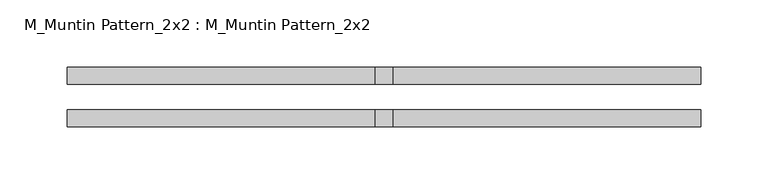
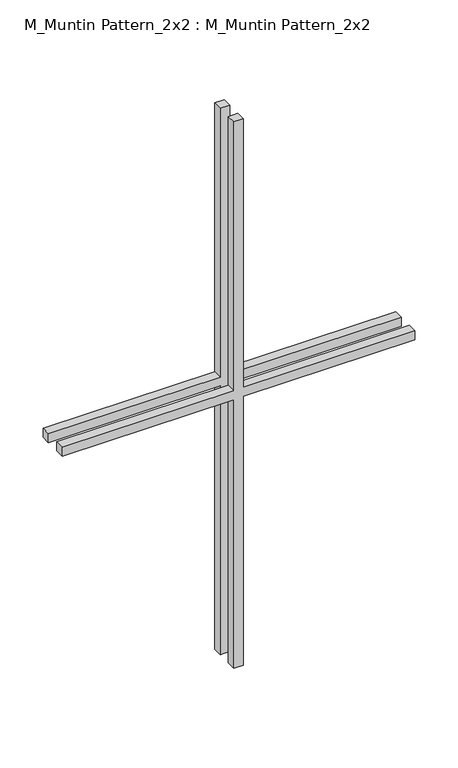
"""IFC4 building model written with IfcOpenShell, lengths in millimetres: proxy geometry, M_Muntin Pattern_2x2 : M_Muntin Pattern_2x2."""

from ifc_helpers import new_model, si_unit, frame, origin, place, context, project, spatial, polyline, outline, extrude, source, transform, mapped, element, save


def m_muntin_pattern_2x2_m_muntin_pattern_2x2_302d8f29(model_context):
    return source(origin(), model_context, "Body", "SweptSolid", [
        extrude(outline(polyline([(393.7, -6.35), (393.7, -236.5375), (381.0, -236.5375), (381.0, -6.35), (0.0, -6.35), (0.0, 6.35), (381.0, 6.35), (381.0, 236.5375), (393.7, 236.5375), (393.7, 6.35), (774.7, 6.35), (774.7, -6.35), (393.7, -6.35)])), frame((0.0, -22.225, 0.0), z_axis=(0.0, 1.0, 0.0), x_axis=(0.0, 0.0, 1.0)), (0.0, 0.0, 1.0), 12.7),
        extrude(outline(polyline([(393.7, -6.35), (393.7, -236.5375), (381.0, -236.5375), (381.0, -6.35), (0.0, -6.35), (0.0, 6.35), (381.0, 6.35), (381.0, 236.5375), (393.7, 236.5375), (393.7, 6.35), (774.7, 6.35), (774.7, -6.35), (393.7, -6.35)])), frame((0.0, 9.525, 0.0), z_axis=(0.0, 1.0, 0.0), x_axis=(0.0, 0.0, 1.0)), (0.0, 0.0, 1.0), 12.7),
    ])


if __name__ == "__main__":
    model = new_model("IFC4")
    model_context = context("Model", 3, world=origin())
    ifc_project = project(units=[si_unit("LENGTHUNIT", "METRE", prefix="MILLI")], contexts=[model_context])
    site = spatial("IfcSite", under=ifc_project)
    building = spatial("IfcBuilding", under=site)
    placement = place(None, origin())
    m_muntin_pattern_2x2_m_muntin_pattern_2x2_shape = m_muntin_pattern_2x2_m_muntin_pattern_2x2_302d8f29(model_context)
    element("IfcBuildingElementProxy", 1, Name="M_Muntin Pattern_2x2 : M_Muntin Pattern_2x2", ObjectType="M_Muntin Pattern_2x2 : M_Muntin Pattern_2x2", at=placement, inside=building, context=model_context, shape_type="MappedRepresentation", body=[
        mapped(m_muntin_pattern_2x2_m_muntin_pattern_2x2_shape, transform((0.0, 0.0, 0.0), x_axis=(1.0, 0.0, 0.0), y_axis=(0.0, 1.0, 0.0), z_axis=(0.0, 0.0, 1.0))),
    ])
    save(model, "model.ifc")

# Revit data of these elements
# Type "M_Muntin Pattern_2x2 : M_Muntin Pattern_2x2"
#   Width [instance default] = 3' - 11.24409"
#   Thickness = 0' - 0 1/2"
#   Height [instance default] = 3' - 11.24409"
#   Distance = 0' - 0 3/4"
#   Interior Material [instance default] = none
#   Exterior Material [instance default] = none
#   Default Elevation = 0
# Element 1 (IfcBuildingElementProxy, "M_Muntin Pattern_2x2 : M_Muntin Pattern_2x2")
#   Width = 1' - 6 5/8"
#   Height = 2' - 6 1/2"
#   Interior Material = Wood - Stained
#   Exterior Material = Clad - White
#   Materials on its faces: "Clad - White", "Wood - Stained"
# Materials
#   "Clad - White": class "Wood", colour RGB 242 242 238, transparency 0, Cost = 0
#   "Wood - Stained": class "Wood", colour RGB 224 178 126, transparency 0, Cost = 0
